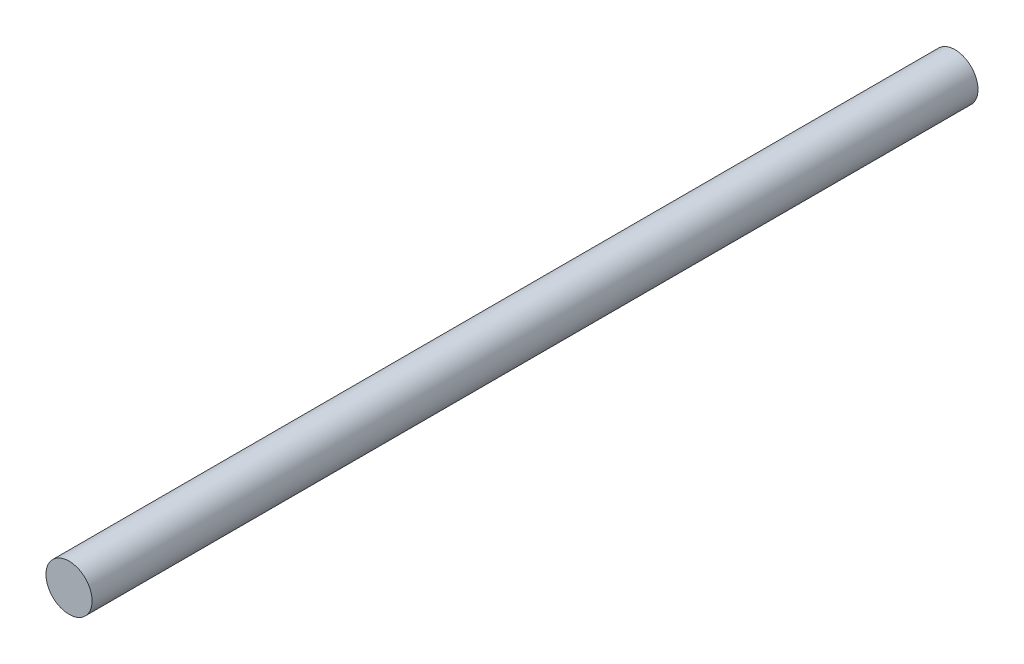
from build123d import *

# Parameters (mm, degrees)
ROD_PROFILE_5_R = 2.5
ROD_5X96_DEPTH  = 48


with BuildPart() as part:
    # Rod Profile Ø5 → Rod Ø5x96 (new, symmetric)
    with BuildSketch(Plane.XY):
        Circle(ROD_PROFILE_5_R)
    extrude(amount=ROD_5X96_DEPTH, both=True)


solid = part.part
